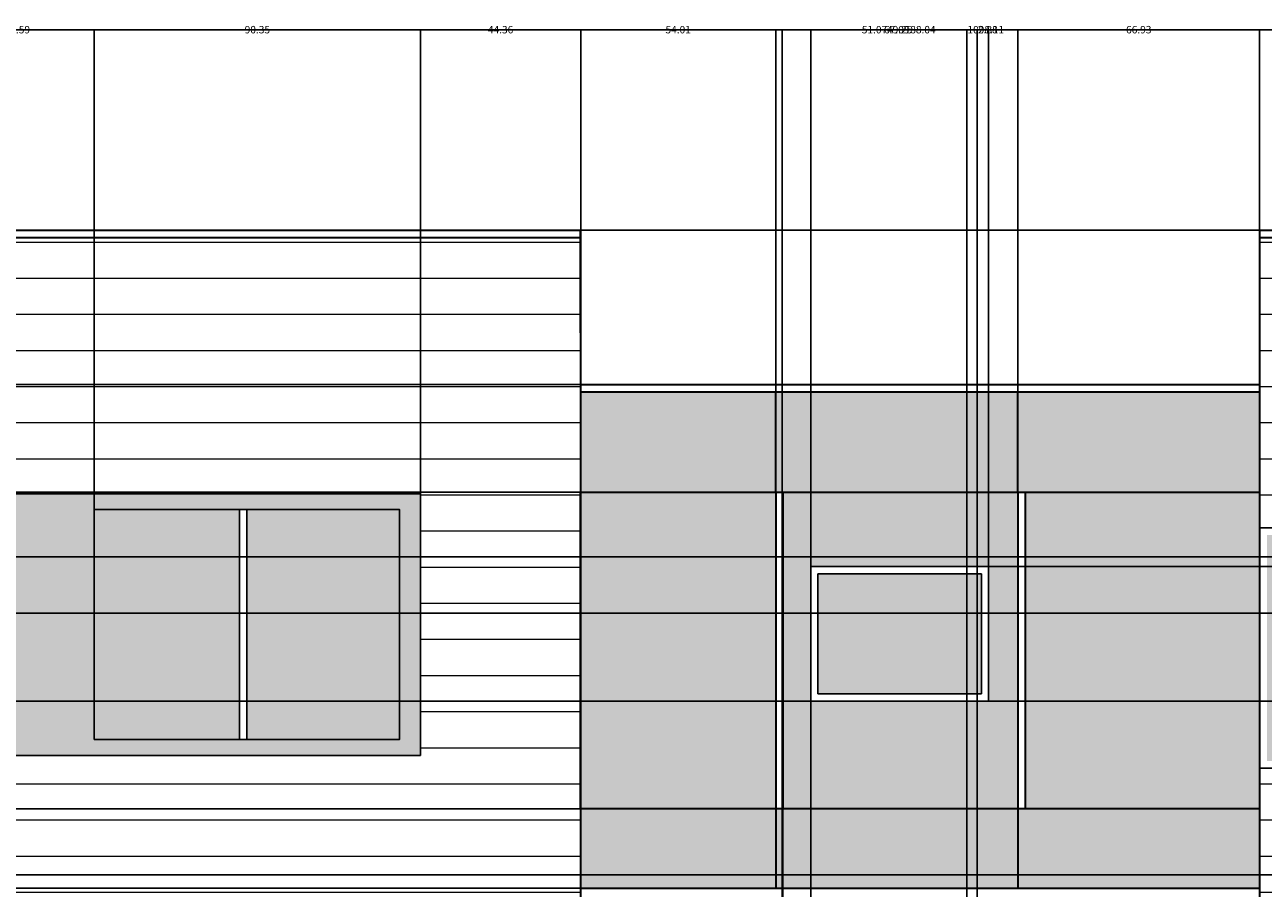
# Model space of a CAD drawing. Units: inches. Extents: x -30 to 1188, y 40 to 520.
# Tile 4 of 7: x 313 to 656, y 281 to 520. Entities that reach past the tile are written whole.
import ezdxf

# ---------------------------------------------------------------- set-up
doc = ezdxf.new("R2010")
doc.units = ezdxf.units.IN
doc.header["$MEASUREMENT"] = 0
for name, color, linetype, lineweight in [('A-ANNO-DIMS', 2, 'Continuous', 18), ('A-ELEV', 7, 'Continuous', 35), ('A-ELEV-PATT', 8, 'Continuous', 13), ('A-GLAZ', 4, 'Continuous', 25)]:
    doc.layers.add(name, color=color, linetype=linetype, lineweight=lineweight)
doc.styles.get("Standard").update_dxf_attribs({"font": 'arial.ttf'})
doc.dimstyles.get("Standard").update_dxf_attribs({"dimtxt": 2.0625, "dimasz": 0.18, "dimexe": 0.18, "dimexo": 0.0625, "dimgap": 0.09, "dimtad": 0, "dimtih": 1, "dimtoh": 1, "dimdec": 4, "dimzin": 0, "dimdsep": 46, "dimlunit": 4, "dimtxsty": 'Standard', "dimcen": 0.09, "dimadec": 0, "dimazin": 0, "dimtfac": 1, "dimtdec": 4, "dimtofl": 0, "dimtmove": 0, "dimatfit": 3, "dimfxl": 1, "dimtolj": 1, "dimtzin": 0, "dimarcsym": 0})

# ---------------------------------------------------------------- blocks, each defined once
blk = doc.blocks.new('WIN-SLIDING')
for p, q in [((40.27, 63.6), (40.27, 0)), ((42.27, 63.6), (42.27, 0))]:
    blk.add_line(p, q)
blk.add_lwpolyline([(0, 63.6), (84.55, 63.6), (84.55, 0), (0, 0)], close=True)
blk = doc.blocks.new('*D5')
at = {"layer": 'A-ANNO-DIMS', "color": 0, "lineweight": -2, "transparency": 16777216}
for p, q in [((73.66, 463.36), (73.66, 518.97)), ((73.84, 518.79), (266.76, 518.79)), ((466.82, 518.79), (273.9, 518.79)), ((467, 463.36), (467, 518.97))]:
    blk.add_line(p, q, dxfattribs=at)
at = {"layer": 'A-ANNO-DIMS', "color": 0, "transparency": 16777216}
for points in [[(73.84, 518.82), (73.84, 518.76), (73.66, 518.79)], [(466.82, 518.82), (466.82, 518.76), (467, 518.79)]]:
    blk.add_solid(points, dxfattribs=at)
at = {"layer": 'Defpoints', "color": 0, "transparency": 16777216}
for p in [(467, 518.79), (73.66, 463.29), (467, 463.29)]:
    blk.add_point(p, dxfattribs=at)
at = {"layer": 'A-ANNO-DIMS', "color": 0, "transparency": 16777216, "insert": (270.33, 518.79), "char_height": 2.062, "attachment_point": 5}
blk.add_mtext('\\A1;393.3', dxfattribs=at)
blk = doc.blocks.new('*D6')
at = {"layer": 'A-ANNO-DIMS', "color": 0, "lineweight": -2, "transparency": 16777216}
for p, q in [((467, 463.36), (467, 518.97)), ((467.18, 518.79), (556.74, 518.79)), ((654.85, 518.79), (565.28, 518.79)), ((655.03, 463.36), (655.03, 518.97))]:
    blk.add_line(p, q, dxfattribs=at)
at = {"layer": 'A-ANNO-DIMS', "color": 0, "transparency": 16777216}
for points in [[(467.18, 518.82), (467.18, 518.76), (467, 518.79)], [(654.85, 518.82), (654.85, 518.76), (655.03, 518.79)]]:
    blk.add_solid(points, dxfattribs=at)
at = {"layer": 'Defpoints', "color": 0, "transparency": 16777216}
for p in [(655.03, 518.79), (467, 463.29), (655.03, 463.29)]:
    blk.add_point(p, dxfattribs=at)
at = {"layer": 'A-ANNO-DIMS', "color": 0, "transparency": 16777216, "insert": (561.01, 518.79), "char_height": 2.062, "attachment_point": 5}
blk.add_mtext('\\A1;188.04', dxfattribs=at)
blk = doc.blocks.new('*D7')
at = {"layer": 'A-ANNO-DIMS', "color": 0, "lineweight": -2, "transparency": 16777216}
for p, q in [((655.03, 463.36), (655.03, 518.97)), ((655.21, 518.79), (791.88, 518.79)), ((935.72, 518.79), (799.06, 518.79)), ((935.9, 463.36), (935.9, 518.97))]:
    blk.add_line(p, q, dxfattribs=at)
at = {"layer": 'A-ANNO-DIMS', "color": 0, "transparency": 16777216}
for points in [[(655.21, 518.82), (655.21, 518.76), (655.03, 518.79)], [(935.72, 518.82), (935.72, 518.76), (935.9, 518.79)]]:
    blk.add_solid(points, dxfattribs=at)
at = {"layer": 'Defpoints', "color": 0, "transparency": 16777216}
for p in [(935.9, 518.79), (655.03, 463.29), (935.9, 463.29)]:
    blk.add_point(p, dxfattribs=at)
at = {"layer": 'A-ANNO-DIMS', "color": 0, "transparency": 16777216, "insert": (795.47, 518.79), "char_height": 2.062, "attachment_point": 5}
blk.add_mtext('\\A1;280.9', dxfattribs=at)
blk = doc.blocks.new('*D15')
at = {"layer": 'A-ANNO-DIMS', "color": 0, "lineweight": -2, "transparency": 16777216}
for p, q in [((289.7, 390.39), (289.7, 518.97)), ((289.88, 518.79), (307.38, 518.79)), ((332.11, 518.79), (314.61, 518.79)), ((332.29, 385.96), (332.29, 518.97))]:
    blk.add_line(p, q, dxfattribs=at)
at = {"layer": 'A-ANNO-DIMS', "color": 0, "transparency": 16777216}
for points in [[(289.88, 518.82), (289.88, 518.76), (289.7, 518.79)], [(332.11, 518.82), (332.11, 518.76), (332.29, 518.79)]]:
    blk.add_solid(points, dxfattribs=at)
at = {"layer": 'Defpoints', "color": 0, "transparency": 16777216}
for p in [(332.29, 518.79), (289.7, 390.32), (332.29, 385.9)]:
    blk.add_point(p, dxfattribs=at)
at = {"layer": 'A-ANNO-DIMS', "color": 0, "transparency": 16777216, "insert": (310.99, 518.79), "char_height": 2.062, "attachment_point": 5}
blk.add_mtext('\\A1;42.59', dxfattribs=at)
blk = doc.blocks.new('*D16')
at = {"layer": 'A-ANNO-DIMS', "color": 0, "lineweight": -2, "transparency": 16777216}
for p, q in [((332.29, 385.96), (332.29, 518.97)), ((332.47, 518.79), (373.89, 518.79)), ((422.46, 518.79), (381.04, 518.79)), ((422.64, 390.39), (422.64, 518.97))]:
    blk.add_line(p, q, dxfattribs=at)
at = {"layer": 'A-ANNO-DIMS', "color": 0, "transparency": 16777216}
for points in [[(332.47, 518.82), (332.47, 518.76), (332.29, 518.79)], [(422.46, 518.82), (422.46, 518.76), (422.64, 518.79)]]:
    blk.add_solid(points, dxfattribs=at)
at = {"layer": 'Defpoints', "color": 0, "transparency": 16777216}
for p in [(422.64, 518.79), (422.64, 390.32), (332.29, 385.9)]:
    blk.add_point(p, dxfattribs=at)
at = {"layer": 'A-ANNO-DIMS', "color": 0, "transparency": 16777216, "insert": (377.46, 518.79), "char_height": 2.062, "attachment_point": 5}
blk.add_mtext('\\A1;90.35', dxfattribs=at)
blk = doc.blocks.new('*D17')
at = {"layer": 'A-ANNO-DIMS', "color": 0, "lineweight": -2, "transparency": 16777216}
for p, q in [((422.64, 390.39), (422.64, 518.97)), ((422.82, 518.79), (441.21, 518.79)), ((466.82, 518.79), (448.43, 518.79)), ((467, 390.84), (467, 518.97))]:
    blk.add_line(p, q, dxfattribs=at)
at = {"layer": 'A-ANNO-DIMS', "color": 0, "transparency": 16777216}
for points in [[(422.82, 518.82), (422.82, 518.76), (422.64, 518.79)], [(466.82, 518.82), (466.82, 518.76), (467, 518.79)]]:
    blk.add_solid(points, dxfattribs=at)
at = {"layer": 'Defpoints', "color": 0, "transparency": 16777216}
for p in [(467, 518.79), (422.64, 390.32), (467, 390.77)]:
    blk.add_point(p, dxfattribs=at)
at = {"layer": 'A-ANNO-DIMS', "color": 0, "transparency": 16777216, "insert": (444.82, 518.79), "char_height": 2.062, "attachment_point": 5}
blk.add_mtext('\\A1;44.36', dxfattribs=at)
blk = doc.blocks.new('*D24')
at = {"layer": 'A-ANNO-DIMS', "color": 0, "lineweight": -2, "transparency": 16777216}
for p, q in [((935.84, 463.29), (-25.83, 463.29)), ((-25.65, 463.11), (-25.65, 419.2)), ((-25.65, 373.01), (-25.65, 416.92)), ((980.66, 372.83), (-25.83, 372.83))]:
    blk.add_line(p, q, dxfattribs=at)
at = {"layer": 'A-ANNO-DIMS', "color": 0, "transparency": 16777216}
for points in [[(-25.68, 463.11), (-25.62, 463.11), (-25.65, 463.29)], [(-25.68, 373.01), (-25.62, 373.01), (-25.65, 372.83)]]:
    blk.add_solid(points, dxfattribs=at)
at = {"layer": 'Defpoints', "color": 0, "transparency": 16777216}
for p in [(-25.65, 463.29), (935.9, 463.29), (980.73, 372.83)]:
    blk.add_point(p, dxfattribs=at)
at = {"layer": 'A-ANNO-DIMS', "color": 0, "transparency": 16777216, "insert": (-25.65, 418.06), "char_height": 2.062, "attachment_point": 5}
blk.add_mtext('\\A1;90.47', dxfattribs=at)
blk = doc.blocks.new('*D25')
at = {"layer": 'A-ANNO-DIMS', "color": 0, "lineweight": -2, "transparency": 16777216}
for p, q in [((655.03, 380.92), (655.03, 518.97)), ((655.21, 518.79), (722.39, 518.79)), ((798.12, 518.79), (730.94, 518.79)), ((798.3, 380.92), (798.3, 518.97))]:
    blk.add_line(p, q, dxfattribs=at)
at = {"layer": 'A-ANNO-DIMS', "color": 0, "transparency": 16777216}
for points in [[(655.21, 518.82), (655.21, 518.76), (655.03, 518.79)], [(798.12, 518.82), (798.12, 518.76), (798.3, 518.79)]]:
    blk.add_solid(points, dxfattribs=at)
at = {"layer": 'Defpoints', "color": 0, "transparency": 16777216}
for p in [(798.3, 518.79), (655.03, 380.86), (798.3, 380.86)]:
    blk.add_point(p, dxfattribs=at)
at = {"layer": 'A-ANNO-DIMS', "color": 0, "transparency": 16777216, "insert": (726.67, 518.79), "char_height": 2.062, "attachment_point": 5}
blk.add_mtext('\\A1;143.27', dxfattribs=at)
blk = doc.blocks.new('*D41')
at = {"layer": 'A-ANNO-DIMS', "color": 0, "lineweight": -2, "transparency": 16777216}
for p, q in [((654.97, 463.29), (-25.83, 463.29)), ((-25.65, 463.11), (-25.65, 443.04)), ((-25.65, 420.69), (-25.65, 440.76)), ((654.97, 420.51), (-25.83, 420.51))]:
    blk.add_line(p, q, dxfattribs=at)
at = {"layer": 'A-ANNO-DIMS', "color": 0, "transparency": 16777216}
for points in [[(-25.68, 463.11), (-25.62, 463.11), (-25.65, 463.29)], [(-25.68, 420.69), (-25.62, 420.69), (-25.65, 420.51)]]:
    blk.add_solid(points, dxfattribs=at)
at = {"layer": 'Defpoints', "color": 0, "transparency": 16777216}
for p in [(655.03, 463.29), (-25.65, 420.51), (655.03, 420.51)]:
    blk.add_point(p, dxfattribs=at)
at = {"layer": 'A-ANNO-DIMS', "color": 0, "transparency": 16777216, "insert": (-25.65, 441.9), "char_height": 2.062, "attachment_point": 5}
blk.add_mtext('\\A1;42.785', dxfattribs=at)
blk = doc.blocks.new('*D45')
at = {"layer": 'A-ANNO-DIMS', "color": 0, "lineweight": -2, "transparency": 16777216}
for p, q in [((945.03, 284.84), (-25.83, 284.84)), ((-25.65, 284.66), (-25.65, 273.81)), ((-25.65, 260.67), (-25.65, 271.52)), ((935.84, 260.49), (-25.83, 260.49))]:
    blk.add_line(p, q, dxfattribs=at)
at = {"layer": 'A-ANNO-DIMS', "color": 0, "transparency": 16777216}
for points in [[(-25.68, 284.66), (-25.62, 284.66), (-25.65, 284.84)], [(-25.68, 260.67), (-25.62, 260.67), (-25.65, 260.49)]]:
    blk.add_solid(points, dxfattribs=at)
at = {"layer": 'Defpoints', "color": 0, "transparency": 16777216}
for p in [(945.1, 284.84), (-25.65, 260.49), (935.9, 260.49)]:
    blk.add_point(p, dxfattribs=at)
at = {"layer": 'A-ANNO-DIMS', "color": 0, "transparency": 16777216, "insert": (-25.65, 272.67), "char_height": 2.062, "attachment_point": 5}
blk.add_mtext('\\A1;24.35', dxfattribs=at)
blk = doc.blocks.new('*D46')
at = {"layer": 'A-ANNO-DIMS', "color": 0, "lineweight": -2, "transparency": 16777216}
for p, q in [((945.03, 357.27), (-25.83, 357.27)), ((-25.65, 357.09), (-25.65, 322.2)), ((-25.65, 285.02), (-25.65, 319.91)), ((945.03, 284.84), (-25.83, 284.84))]:
    blk.add_line(p, q, dxfattribs=at)
at = {"layer": 'A-ANNO-DIMS', "color": 0, "transparency": 16777216}
for points in [[(-25.68, 357.09), (-25.62, 357.09), (-25.65, 357.27)], [(-25.68, 285.02), (-25.62, 285.02), (-25.65, 284.84)]]:
    blk.add_solid(points, dxfattribs=at)
at = {"layer": 'Defpoints', "color": 0, "transparency": 16777216}
for p in [(-25.65, 357.27), (945.1, 357.27), (945.1, 284.84)]:
    blk.add_point(p, dxfattribs=at)
at = {"layer": 'A-ANNO-DIMS', "color": 0, "transparency": 16777216, "insert": (-25.65, 321.06), "char_height": 2.062, "attachment_point": 5}
blk.add_mtext('\\A1;72.43', dxfattribs=at)
blk = doc.blocks.new('*D47')
at = {"layer": 'A-ANNO-DIMS', "color": 0, "lineweight": -2, "transparency": 16777216}
for p, q in [((935.84, 372.83), (-25.83, 372.83)), ((-25.65, 372.65), (-25.65, 366.19)), ((-25.65, 357.45), (-25.65, 363.91)), ((945.03, 357.27), (-25.83, 357.27))]:
    blk.add_line(p, q, dxfattribs=at)
at = {"layer": 'A-ANNO-DIMS', "color": 0, "transparency": 16777216}
for points in [[(-25.68, 372.65), (-25.62, 372.65), (-25.65, 372.83)], [(-25.68, 357.45), (-25.62, 357.45), (-25.65, 357.27)]]:
    blk.add_solid(points, dxfattribs=at)
at = {"layer": 'Defpoints', "color": 0, "transparency": 16777216}
for p in [(-25.65, 372.83), (935.9, 372.83), (945.1, 357.27)]:
    blk.add_point(p, dxfattribs=at)
at = {"layer": 'A-ANNO-DIMS', "color": 0, "transparency": 16777216, "insert": (-25.65, 365.05), "char_height": 2.062, "attachment_point": 5}
blk.add_mtext('\\A1;15.554', dxfattribs=at)
blk = doc.blocks.new('*D58')
at = {"layer": 'A-ANNO-DIMS', "color": 0, "lineweight": -2, "transparency": 16777216}
for p, q in [((466.93, 303.05), (-25.83, 303.05)), ((-25.65, 302.87), (-25.65, 293.22)), ((-25.65, 281.27), (-25.65, 290.93)), ((466.93, 281.09), (-25.83, 281.09))]:
    blk.add_line(p, q, dxfattribs=at)
at = {"layer": 'A-ANNO-DIMS', "color": 0, "transparency": 16777216}
for points in [[(-25.68, 302.87), (-25.62, 302.87), (-25.65, 303.05)], [(-25.68, 281.27), (-25.62, 281.27), (-25.65, 281.09)]]:
    blk.add_solid(points, dxfattribs=at)
at = {"layer": 'Defpoints', "color": 0, "transparency": 16777216}
for p in [(-25.65, 303.05), (467, 303.05), (467, 281.09)]:
    blk.add_point(p, dxfattribs=at)
at = {"layer": 'A-ANNO-DIMS', "color": 0, "transparency": 16777216, "insert": (-25.65, 292.07), "char_height": 2.062, "attachment_point": 5}
blk.add_mtext('\\A1;21.96', dxfattribs=at)
blk = doc.blocks.new('*D59')
at = {"layer": 'A-ANNO-DIMS', "color": 0, "lineweight": -2, "transparency": 16777216}
for p, q in [((466.93, 390.77), (-25.83, 390.77)), ((-25.65, 390.59), (-25.65, 348.06)), ((-25.65, 303.23), (-25.65, 345.77)), ((466.93, 303.05), (-25.83, 303.05))]:
    blk.add_line(p, q, dxfattribs=at)
at = {"layer": 'A-ANNO-DIMS', "color": 0, "transparency": 16777216}
for points in [[(-25.68, 390.59), (-25.62, 390.59), (-25.65, 390.77)], [(-25.68, 303.23), (-25.62, 303.23), (-25.65, 303.05)]]:
    blk.add_solid(points, dxfattribs=at)
at = {"layer": 'Defpoints', "color": 0, "transparency": 16777216}
for p in [(-25.65, 390.77), (467, 390.77), (467, 303.05)]:
    blk.add_point(p, dxfattribs=at)
at = {"layer": 'A-ANNO-DIMS', "color": 0, "transparency": 16777216, "insert": (-25.65, 346.91), "char_height": 2.062, "attachment_point": 5}
blk.add_mtext('\\A1;87.72', dxfattribs=at)
blk = doc.blocks.new('*D60')
at = {"layer": 'A-ANNO-DIMS', "color": 0, "lineweight": -2, "transparency": 16777216}
for p, q in [((466.93, 420.51), (-25.83, 420.51)), ((-25.65, 420.33), (-25.65, 406.78)), ((-25.65, 390.95), (-25.65, 404.5)), ((466.93, 390.77), (-25.83, 390.77))]:
    blk.add_line(p, q, dxfattribs=at)
at = {"layer": 'A-ANNO-DIMS', "color": 0, "transparency": 16777216}
for points in [[(-25.68, 420.33), (-25.62, 420.33), (-25.65, 420.51)], [(-25.68, 390.95), (-25.62, 390.95), (-25.65, 390.77)]]:
    blk.add_solid(points, dxfattribs=at)
at = {"layer": 'Defpoints', "color": 0, "transparency": 16777216}
for p in [(-25.65, 420.51), (467, 420.51), (467, 390.77)]:
    blk.add_point(p, dxfattribs=at)
at = {"layer": 'A-ANNO-DIMS', "color": 0, "transparency": 16777216, "insert": (-25.65, 405.64), "char_height": 2.062, "attachment_point": 5}
blk.add_mtext('\\A1;29.735', dxfattribs=at)
blk = doc.blocks.new('*D65')
at = {"layer": 'A-ANNO-DIMS', "color": 0, "lineweight": -2, "transparency": 16777216}
for p, q in [((522.84, 271.44), (522.84, 518.97)), ((523.02, 518.79), (544.8, 518.79)), ((573.72, 518.79), (551.94, 518.79)), ((573.9, 245.23), (573.9, 518.97))]:
    blk.add_line(p, q, dxfattribs=at)
at = {"layer": 'A-ANNO-DIMS', "color": 0, "transparency": 16777216}
for points in [[(523.02, 518.82), (523.02, 518.76), (522.84, 518.79)], [(573.72, 518.82), (573.72, 518.76), (573.9, 518.79)]]:
    blk.add_solid(points, dxfattribs=at)
at = {"layer": 'Defpoints', "color": 0, "transparency": 16777216}
for p in [(522.84, 518.79), (522.84, 271.38), (573.9, 245.17)]:
    blk.add_point(p, dxfattribs=at)
at = {"layer": 'A-ANNO-DIMS', "color": 0, "transparency": 16777216, "insert": (548.37, 518.79), "char_height": 2.062, "attachment_point": 5}
blk.add_mtext('\\A1;51.07', dxfattribs=at)
blk = doc.blocks.new('*D66')
at = {"layer": 'A-ANNO-DIMS', "color": 0, "lineweight": -2, "transparency": 16777216}
for p, q in [((573.9, 245.23), (573.9, 518.97)), ((574.08, 518.79), (576.6, 518.79)), ((576.78, 245.23), (576.78, 518.97)), ((576.78, 518.79), (576.96, 518.79))]:
    blk.add_line(p, q, dxfattribs=at)
at = {"layer": 'A-ANNO-DIMS', "color": 0, "transparency": 16777216}
for points in [[(574.08, 518.82), (574.08, 518.76), (573.9, 518.79)], [(576.6, 518.82), (576.6, 518.76), (576.78, 518.79)]]:
    blk.add_solid(points, dxfattribs=at)
at = {"layer": 'Defpoints', "color": 0, "transparency": 16777216}
for p in [(576.78, 518.79), (573.9, 245.17), (576.78, 245.17)]:
    blk.add_point(p, dxfattribs=at)
at = {"layer": 'A-ANNO-DIMS', "color": 0, "transparency": 16777216, "insert": (579.75, 518.79), "char_height": 2.062, "attachment_point": 5}
blk.add_mtext('\\A1;2.88', dxfattribs=at)
blk = doc.blocks.new('*D67')
at = {"layer": 'A-ANNO-DIMS', "color": 0, "lineweight": -2, "transparency": 16777216}
for p, q in [((530.73, 370.19), (530.73, 518.97)), ((530.91, 518.79), (551.73, 518.79)), ((579.79, 518.79), (558.97, 518.79)), ((579.97, 370.19), (579.97, 518.97))]:
    blk.add_line(p, q, dxfattribs=at)
at = {"layer": 'A-ANNO-DIMS', "color": 0, "transparency": 16777216}
for points in [[(530.91, 518.82), (530.91, 518.76), (530.73, 518.79)], [(579.79, 518.82), (579.79, 518.76), (579.97, 518.79)]]:
    blk.add_solid(points, dxfattribs=at)
at = {"layer": 'Defpoints', "color": 0, "transparency": 16777216}
for p in [(579.97, 518.79), (530.73, 370.13), (579.97, 370.13)]:
    blk.add_point(p, dxfattribs=at)
at = {"layer": 'A-ANNO-DIMS', "color": 0, "transparency": 16777216, "insert": (555.35, 518.79), "char_height": 2.062, "attachment_point": 5}
blk.add_mtext('\\A1;49.25', dxfattribs=at)
blk = doc.blocks.new('*D68')
at = {"layer": 'A-ANNO-DIMS', "color": 0, "lineweight": -2, "transparency": 16777216}
for p, q in [((580.04, 370.13), (1183.93, 370.13)), ((1183.75, 369.95), (1183.75, 352.67)), ((1183.75, 333.09), (1183.75, 350.38)), ((580.04, 332.91), (1183.93, 332.91))]:
    blk.add_line(p, q, dxfattribs=at)
at = {"layer": 'A-ANNO-DIMS', "color": 0, "transparency": 16777216}
for points in [[(1183.72, 369.95), (1183.78, 369.95), (1183.75, 370.13)], [(1183.72, 333.09), (1183.78, 333.09), (1183.75, 332.91)]]:
    blk.add_solid(points, dxfattribs=at)
at = {"layer": 'Defpoints', "color": 0, "transparency": 16777216}
for p in [(579.97, 370.13), (1183.75, 370.13), (579.97, 332.91)]:
    blk.add_point(p, dxfattribs=at)
at = {"layer": 'A-ANNO-DIMS', "color": 0, "transparency": 16777216, "insert": (1183.75, 351.52), "char_height": 2.062, "attachment_point": 5}
blk.add_mtext('\\A1;37.22', dxfattribs=at)
blk = doc.blocks.new('*D69')
at = {"layer": 'A-ANNO-DIMS', "color": 0, "lineweight": -2, "transparency": 16777216}
for p, q in [((530.66, 332.91), (-25.83, 332.91)), ((-25.65, 332.73), (-25.65, 319.13)), ((-25.65, 303.23), (-25.65, 316.84)), ((520.94, 303.05), (-25.83, 303.05))]:
    blk.add_line(p, q, dxfattribs=at)
at = {"layer": 'A-ANNO-DIMS', "color": 0, "transparency": 16777216}
for points in [[(-25.68, 332.73), (-25.62, 332.73), (-25.65, 332.91)], [(-25.68, 303.23), (-25.62, 303.23), (-25.65, 303.05)]]:
    blk.add_solid(points, dxfattribs=at)
at = {"layer": 'Defpoints', "color": 0, "transparency": 16777216}
for p in [(-25.65, 332.91), (530.73, 332.91), (521.01, 303.05)]:
    blk.add_point(p, dxfattribs=at)
at = {"layer": 'A-ANNO-DIMS', "color": 0, "transparency": 16777216, "insert": (-25.65, 317.98), "char_height": 2.062, "attachment_point": 5}
blk.add_mtext('\\A1;29.86', dxfattribs=at)
blk = doc.blocks.new('*D70')
at = {"layer": 'A-ANNO-DIMS', "color": 0, "lineweight": -2, "transparency": 16777216}
for p, q in [((530.73, 332.85), (530.73, 41.19)), ((523.01, 302.99), (523.01, 41.19)), ((523.19, 41.37), (523.3, 41.37)), ((530.55, 41.37), (530.43, 41.37))]:
    blk.add_line(p, q, dxfattribs=at)
at = {"layer": 'A-ANNO-DIMS', "color": 0, "transparency": 16777216}
for points in [[(523.19, 41.4), (523.19, 41.34), (523.01, 41.37)], [(530.55, 41.4), (530.55, 41.34), (530.73, 41.37)]]:
    blk.add_solid(points, dxfattribs=at)
at = {"layer": 'Defpoints', "color": 0, "transparency": 16777216}
for p in [(530.73, 332.91), (523.01, 303.05), (523.01, 41.37)]:
    blk.add_point(p, dxfattribs=at)
at = {"layer": 'A-ANNO-DIMS', "color": 0, "transparency": 16777216, "insert": (526.87, 41.37), "char_height": 2.062, "attachment_point": 5}
blk.add_mtext('\\A1;7.718', dxfattribs=at)
blk = doc.blocks.new('*D71')
at = {"layer": 'A-ANNO-DIMS', "color": 0, "lineweight": -2, "transparency": 16777216}
for p, q in [((467, 418.57), (467, 518.97)), ((467.18, 518.79), (490.63, 518.79)), ((520.83, 518.79), (497.37, 518.79)), ((521.01, 418.57), (521.01, 518.97))]:
    blk.add_line(p, q, dxfattribs=at)
at = {"layer": 'A-ANNO-DIMS', "color": 0, "transparency": 16777216}
for points in [[(467.18, 518.82), (467.18, 518.76), (467, 518.79)], [(520.83, 518.82), (520.83, 518.76), (521.01, 518.79)]]:
    blk.add_solid(points, dxfattribs=at)
at = {"layer": 'Defpoints', "color": 0, "transparency": 16777216}
for p in [(521.01, 518.79), (467, 418.51), (521.01, 418.51)]:
    blk.add_point(p, dxfattribs=at)
at = {"layer": 'A-ANNO-DIMS', "color": 0, "transparency": 16777216, "insert": (494, 518.79), "char_height": 2.062, "attachment_point": 5}
blk.add_mtext('\\A1;54.01', dxfattribs=at)
blk = doc.blocks.new('*D72')
at = {"layer": 'A-ANNO-DIMS', "color": 0, "lineweight": -2, "transparency": 16777216}
for p, q in [((521.01, 418.57), (521.01, 518.97)), ((521.19, 518.79), (550.97, 518.79)), ((587.92, 518.79), (558.13, 518.79)), ((588.1, 418.57), (588.1, 518.97))]:
    blk.add_line(p, q, dxfattribs=at)
at = {"layer": 'A-ANNO-DIMS', "color": 0, "transparency": 16777216}
for points in [[(521.19, 518.82), (521.19, 518.76), (521.01, 518.79)], [(587.92, 518.82), (587.92, 518.76), (588.1, 518.79)]]:
    blk.add_solid(points, dxfattribs=at)
at = {"layer": 'Defpoints', "color": 0, "transparency": 16777216}
for p in [(588.1, 518.79), (521.01, 418.51), (588.1, 418.51)]:
    blk.add_point(p, dxfattribs=at)
at = {"layer": 'A-ANNO-DIMS', "color": 0, "transparency": 16777216, "insert": (554.55, 518.79), "char_height": 2.062, "attachment_point": 5}
blk.add_mtext('\\A1;67.09', dxfattribs=at)
blk = doc.blocks.new('*D73')
at = {"layer": 'A-ANNO-DIMS', "color": 0, "lineweight": -2, "transparency": 16777216}
for p, q in [((588.1, 418.57), (588.1, 518.97)), ((588.28, 518.79), (617.99, 518.79)), ((654.85, 518.79), (625.14, 518.79)), ((655.03, 418.57), (655.03, 518.97))]:
    blk.add_line(p, q, dxfattribs=at)
at = {"layer": 'A-ANNO-DIMS', "color": 0, "transparency": 16777216}
for points in [[(588.28, 518.82), (588.28, 518.76), (588.1, 518.79)], [(654.85, 518.82), (654.85, 518.76), (655.03, 518.79)]]:
    blk.add_solid(points, dxfattribs=at)
at = {"layer": 'Defpoints', "color": 0, "transparency": 16777216}
for p in [(655.03, 518.79), (588.1, 418.51), (655.03, 418.51)]:
    blk.add_point(p, dxfattribs=at)
at = {"layer": 'A-ANNO-DIMS', "color": 0, "transparency": 16777216, "insert": (621.56, 518.79), "char_height": 2.062, "attachment_point": 5}
blk.add_mtext('\\A1;66.93', dxfattribs=at)
blk = doc.blocks.new('*D74')
at = {"layer": 'A-ANNO-DIMS', "color": 0, "lineweight": -2, "transparency": 16777216}
for p, q in [((30.14, 98.93), (30.14, 518.97)), ((30.32, 518.79), (574.32, 518.79)), ((1128.07, 518.79), (584.07, 518.79)), ((1128.25, 117.62), (1128.25, 518.97))]:
    blk.add_line(p, q, dxfattribs=at)
at = {"layer": 'A-ANNO-DIMS', "color": 0, "transparency": 16777216}
for points in [[(30.32, 518.82), (30.32, 518.76), (30.14, 518.79)], [(1128.07, 518.82), (1128.07, 518.76), (1128.25, 518.79)]]:
    blk.add_solid(points, dxfattribs=at)
at = {"layer": 'Defpoints', "color": 0, "transparency": 16777216}
for p in [(1128.25, 518.79), (1128.25, 117.56), (30.14, 98.87)]:
    blk.add_point(p, dxfattribs=at)
at = {"layer": 'A-ANNO-DIMS', "color": 0, "transparency": 16777216, "insert": (579.19, 518.79), "char_height": 2.0625, "attachment_point": 5}
blk.add_mtext('\\A1;1098.11', dxfattribs=at)

msp = doc.modelspace()

# ---------------------------------------------------------------- hatches: boundary and pattern name
at = {"layer": 'A-ELEV-PATT'}
h = msp.add_hatch(dxfattribs=at)
h.set_pattern_fill('ANSI31', color=256, scale=80, angle=135)
h.paths.add_polyline_path([(935.904, 461.2934), (655.0318, 461.2934), (655.0318, 408.0708), (655.0318, 380.8615), (798.3036, 380.8615), (798.3036, 314.3348), (655.0318, 314.3348), (655.0318, 303.0545), (655.0318, 122.8714), (744.4225, 122.8714), (796.5546, 122.8714), (935.904, 122.8714), (935.904, 203.8438), (792.6322, 203.8438), (792.6322, 270.3705), (935.904, 270.3705), (935.904, 372.8284)])
h.paths.add_polyline_path([(466.9951, 434.8714), (466.9951, 461.2934), (73.6582, 461.2934), (73.6582, 434.8714), (73.6582, 410.8714), (73.6582, 266.8714), (382.4247, 266.8714), (466.9951, 266.8714)])
h.paths.add_polyline_path([(422.6392, 390.3227), (422.6392, 317.8826), (99.4312, 317.8826), (99.4312, 390.3227)], flags=16)
h.paths.add_polyline_path([(416.8376, 385.9009), (416.8376, 322.3026), (332.2885, 322.3026), (332.2885, 385.9009)], flags=0)
h.paths.add_polyline_path([(187.4151, 386.0591), (187.4151, 322.4608), (102.866, 322.4608), (102.866, 386.0591)], flags=0)
h = msp.add_hatch(color=256, dxfattribs=at)
h.dxf.hatch_style = 1
h.paths.add_polyline_path([(99.4312, 186.9265), (73.6582, 186.9265), (73.6582, 133.1393), (99.4312, 133.1393)])
h.paths.add_polyline_path([(99.4312, 242.8714), (73.6582, 242.8714), (73.6582, 186.9265), (99.4312, 186.9265)])
h.paths.add_polyline_path([(99.4312, 266.8714), (73.6582, 266.8714), (73.6582, 242.8714), (99.4312, 242.8714)])
h.paths.add_polyline_path([(244.2768, 266.8714), (99.4312, 266.8714), (99.4312, 242.8714), (130.129, 242.8714), (244.2768, 242.8714)])
h.paths.add_polyline_path([(358.4247, 266.8714), (244.2768, 266.8714), (244.2768, 242.8714), (358.4247, 242.8714)])
h.paths.add_polyline_path([(466.8255, 266.8714), (382.4247, 266.8714), (358.4247, 266.8714), (358.4247, 242.8714), (382.4247, 242.8714), (466.8255, 242.8714)])
h.paths.add_polyline_path([(466.8255, 242.8714), (382.4247, 242.8714), (358.4247, 242.8714), (358.4247, 186.9265), (382.4247, 186.9265), (466.8255, 186.9265)])
h.paths.add_polyline_path([(466.8255, 186.9265), (382.4247, 186.9265), (358.4247, 186.9265), (358.4247, 133.1393), (382.4247, 133.1393), (466.9951, 133.1393), (466.9951, 140.7981), (466.8255, 140.7981)])
h.paths.add_polyline_path([(521.0073, 303.0545), (466.9951, 303.0545), (466.9951, 281.0934), (521.0073, 281.0934)])
h.paths.add_polyline_path([(588.0971, 303.0545), (521.0073, 303.0545), (521.0073, 281.0934), (588.0971, 281.0934)])
h.paths.add_polyline_path([(655.0318, 303.0545), (588.0971, 303.0545), (588.0971, 281.0934), (655.0318, 281.0934)])
h.paths.add_polyline_path([(655.0318, 408.0708), (655.0318, 418.5083), (588.0971, 418.5083), (588.0971, 390.7733), (655.0318, 390.7733)])
h.paths.add_polyline_path([(588.0971, 418.5083), (521.0073, 418.5083), (521.0073, 390.7733), (588.0971, 390.7733)])
h.paths.add_polyline_path([(521.0073, 418.5083), (466.9951, 418.5083), (466.9951, 390.7733), (521.0073, 390.7733)])
h = msp.add_hatch(color=256, dxfattribs=at)
h.dxf.hatch_style = 1
h.paths.add_polyline_path([(521.0073, 390.7733), (466.9951, 390.7733), (466.9951, 303.0545), (521.0073, 303.0545)])
h.paths.add_polyline_path([(588.0971, 390.7733), (523.0073, 390.7733), (523.0073, 303.0545), (588.0971, 303.0545)])
h.paths.add_polyline_path([(579.9749, 370.1304), (579.9749, 332.9128), (530.7254, 332.9128), (530.7254, 370.1304)], flags=16)
h.paths.add_polyline_path([(577.9749, 368.1304), (577.9749, 334.9128), (532.7254, 334.9128), (532.7254, 368.1304)], flags=0)
h.paths.add_polyline_path([(655.0318, 390.7733), (590.0971, 390.7733), (590.0971, 303.0545), (655.0318, 303.0545)])
h.paths.add_polyline_path([(577.9749, 368.1304), (532.7254, 368.1304), (532.7254, 334.9128), (577.9749, 334.9128)], flags=0)
h.paths.add_polyline_path([(416.8376, 385.9009), (374.5631, 385.9009), (374.5631, 322.3026), (416.8376, 322.3026)])
h.paths.add_polyline_path([(372.5631, 385.9009), (332.2885, 385.9009), (332.2885, 322.3026), (372.5631, 322.3026)])
h.paths.add_polyline_path([(187.4151, 386.0591), (102.866, 386.0591), (102.866, 322.4608), (187.4151, 322.4608)])
h.paths.add_polyline_path([(697.0557, 378.8615), (657.0318, 378.8615), (657.0318, 316.3348), (697.0557, 316.3348)])
h.paths.add_polyline_path([(746.916, 378.8615), (699.0557, 378.8615), (699.0557, 316.3348), (746.916, 316.3348)])
h.paths.add_polyline_path([(796.3036, 378.8615), (748.916, 378.8615), (748.916, 316.3348), (796.3036, 316.3348)])
h.paths.add_polyline_path([(884.5164, 268.3705), (836.6561, 268.3705), (836.6561, 205.8438), (884.5164, 205.8438)])
h.paths.add_polyline_path([(834.6561, 268.3705), (794.6322, 268.3705), (794.6322, 205.8438), (834.6561, 205.8438)])
h.paths.add_polyline_path([(967.928, 357.2748), (945.0964, 357.2748), (945.0964, 284.8425), (967.928, 284.8425)])
h = msp.add_hatch(color=256, dxfattribs=at)
h.dxf.hatch_style = 1
h.paths.add_polyline_path([(237.1312, 390.3227), (187.4151, 390.3227), (187.4151, 386.0591), (187.4151, 322.4608), (187.4151, 317.8826), (237.1312, 317.8826)])
h.paths.add_polyline_path([(289.6973, 390.3227), (237.1312, 390.3227), (237.1312, 317.8826), (289.6973, 317.8826)])
h.paths.add_polyline_path([(422.6392, 390.3227), (289.6973, 390.3227), (289.6973, 317.8826), (422.6392, 317.8826)])
h.paths.add_polyline_path([(332.2885, 385.9009), (416.8376, 385.9009), (416.8376, 322.3026), (332.2885, 322.3026)], flags=16)
h.paths.add_polyline_path([(520.8377, 255.4488), (468.8255, 255.4488), (468.8255, 208.218), (520.8377, 208.218)])
h.paths.add_polyline_path([(573.9028, 245.1654), (576.7826, 245.1654), (576.7826, 208.218), (587.9675, 208.218), (587.9675, 255.4488), (522.8377, 255.4488), (522.8377, 208.218), (573.9028, 208.218)])
h.paths.add_polyline_path([(652.8622, 255.4488), (589.9675, 255.4488), (589.9675, 208.218), (652.8622, 208.218)])
h.paths.add_polyline_path([(652.8622, 206.218), (589.9675, 206.218), (589.9675, 142.7981), (652.8622, 142.7981)])
h.paths.add_polyline_path([(573.9028, 206.218), (522.8377, 206.218), (522.8377, 142.7981), (587.9675, 142.7981), (587.9675, 206.218), (576.7826, 206.218), (576.7826, 153.0843), (573.9028, 153.0843)])
h.paths.add_polyline_path([(520.8377, 206.218), (468.8255, 206.218), (468.8255, 142.7981), (520.8377, 142.7981)])
h.paths.add_polyline_path([(520.8377, 271.3754), (468.8255, 271.3754), (468.8255, 255.4488), (520.8377, 255.4488)])
h.paths.add_polyline_path([(587.9675, 271.3754), (522.8377, 271.3754), (522.8377, 255.4488), (587.9675, 255.4488)])
h.paths.add_polyline_path([(652.8622, 271.3754), (589.9675, 271.3754), (589.9675, 255.4488), (652.8622, 255.4488)])
h.paths.add_polyline_path([(935.904, 270.3705), (886.5164, 270.3705), (886.5164, 268.3705), (886.5164, 205.8438), (886.5164, 203.8438), (935.904, 203.8438)])
h.paths.add_polyline_path([(978.7252, 275.3408), (937.904, 275.3408), (937.904, 262.4906), (978.7252, 262.4906)])
h.paths.add_polyline_path([(978.7252, 370.8284), (937.904, 370.8284), (937.904, 275.3408), (978.7252, 275.3408)])
h.paths.add_polyline_path([(967.928, 284.8425), (945.0964, 284.8425), (945.0964, 357.2748), (967.928, 357.2748)], flags=16)
h = msp.add_hatch(color=256, dxfattribs=at)
h.dxf.hatch_style = 1
h.paths.add_polyline_path([(577.9749, 368.1304), (532.7254, 368.1304), (532.7254, 334.9128), (577.9749, 334.9128)])

# ---------------------------------------------------------------- linework, layer by layer
at = {"layer": 'A-ELEV'}
for p, q in [((73.6582, 463.2934), (466.9951, 463.2934)), ((466.9951, 434.8714), (466.9951, 463.2934)), ((655.0318, 463.2934), (655.0318, 408.0708)), ((655.0318, 463.2934), (935.904, 463.2934)), ((73.6582, 461.2934), (466.9951, 461.2934)), ((655.0318, 461.2934), (935.904, 461.2934)), ((466.9951, 434.8714), (466.9951, 266.8714)), ((466.9951, 420.5083), (655.0318, 420.5083)), ((466.9951, 418.5083), (655.0318, 418.5083)), ((521.0073, 390.7733), (521.0073, 418.5083)), ((588.0971, 390.7733), (588.0971, 418.5083)), ((655.0318, 408.0708), (655.0318, 122.8714)), ((521.0073, 390.7733), (521.0073, 303.0545)), ((523.0073, 390.7733), (523.0073, 303.0545)), ((588.0971, 390.7733), (588.0971, 303.0545)), ((590.0971, 390.7733), (590.0971, 303.0545)), ((521.0073, 303.0545), (521.0073, 281.0934)), ((588.0971, 303.0545), (588.0971, 281.0934)), ((466.9951, 281.0934), (655.0318, 281.0934))]:
    msp.add_line(p, q, dxfattribs=at)
msp.add_lwpolyline([(466.9951, 390.7733), (655.0318, 390.7733), (655.0318, 303.0545), (466.9951, 303.0545)], close=True, dxfattribs=at)
at = {"layer": 'A-GLAZ'}
for points in [[(99.4312, 390.3227), (422.6392, 390.3227), (422.6392, 317.8826), (99.4312, 317.8826)], [(655.0318, 380.8615), (798.3036, 380.8615), (798.3036, 314.3348), (655.0318, 314.3348)], [(530.7254, 370.1304), (579.9749, 370.1304), (579.9749, 332.9128), (530.7254, 332.9128)], [(532.7254, 368.1304), (577.9749, 368.1304), (577.9749, 334.9128), (532.7254, 334.9128)]]:
    msp.add_lwpolyline(points, close=True, dxfattribs=at)

# ---------------------------------------------------------------- block references
msp.add_blockref('WIN-SLIDING', (332.2886, 322.3028), dxfattribs=at)

# ---------------------------------------------------------------- dimensions: what is measured, and where the dimension line sits
at = {"layer": 'A-ANNO-DIMS'}
for base, p1, p2, override, picture, middle in [((1128.2474, 518.7934), (30.1395, 98.8714), (1128.2474, 117.5588), {"dimdec": 2, "dimlfac": 1, "dimrnd": 0, "dimzin": 0, "dimdsep": 46, "dimlunit": 2}, '*D74', (579.1935, 518.7934)), ((466.9951, 518.7934), (73.6582, 463.2934), (466.9951, 463.2934), {"dimdec": 1, "dimlfac": 1, "dimrnd": 0, "dimzin": 0, "dimdsep": 46, "dimlunit": 2}, '*D5', (270.3266, 518.7934)), ((332.2885, 518.7934), (289.6973, 390.3227), (332.2885, 385.9009), {"dimdec": 2, "dimlfac": 1, "dimrnd": 0, "dimzin": 0, "dimdsep": 46, "dimlunit": 2}, '*D15', (310.9929, 518.7934)), ((422.6392, 518.7934), (332.2885, 385.9009), (422.6392, 390.3227), {"dimdec": 2, "dimlfac": 1, "dimrnd": 0, "dimzin": 0, "dimdsep": 46, "dimlunit": 2}, '*D16', (377.4639, 518.7934)), ((466.9951, 518.7934), (422.6392, 390.3227), (466.9951, 390.7733), {"dimdec": 2, "dimlfac": 1, "dimrnd": 0, "dimzin": 0, "dimdsep": 46, "dimlunit": 2}, '*D17', (444.8171, 518.7934)), ((655.0318, 518.7934), (466.9951, 463.2934), (655.0318, 463.2934), {"dimdec": 2, "dimlfac": 1, "dimrnd": 0, "dimzin": 0, "dimdsep": 46, "dimlunit": 2}, '*D6', (561.0134, 518.7934)), ((521.0073, 518.7934), (466.9951, 418.5083), (521.0073, 418.5083), {"dimdec": 2, "dimlfac": 1, "dimrnd": 0, "dimzin": 0, "dimdsep": 46, "dimlunit": 2}, '*D71', (494.0012, 518.7934)), ((588.0971, 518.7934), (521.0073, 418.5083), (588.0971, 418.5083), {"dimdec": 2, "dimlfac": 1, "dimrnd": 0, "dimzin": 0, "dimdsep": 46, "dimlunit": 2}, '*D72', (554.5522, 518.7934)), ((522.8377, 518.7934), (573.9028, 245.1654), (522.8377, 271.3754), {"dimdec": 2, "dimlfac": 1, "dimrnd": 0, "dimzin": 0, "dimdsep": 46, "dimlunit": 2}, '*D65', (548.3702, 518.7934)), ((579.9749, 518.7934), (530.7254, 370.1304), (579.9749, 370.1304), {"dimdec": 2, "dimlfac": 1, "dimrnd": 0, "dimzin": 0, "dimdsep": 46, "dimlunit": 2}, '*D67', (555.3501, 518.7934)), ((576.7826, 518.7934), (573.9028, 245.1654), (576.7826, 245.1654), {"dimdec": 2, "dimlfac": 1, "dimrnd": 0, "dimzin": 0, "dimdsep": 46, "dimlunit": 2}, '*D66', (579.751, 518.7934)), ((655.0318, 518.7934), (588.0971, 418.5083), (655.0318, 418.5083), {"dimdec": 2, "dimlfac": 1, "dimrnd": 0, "dimzin": 0, "dimdsep": 46, "dimlunit": 2}, '*D73', (621.5645, 518.7934)), ((935.904, 518.7934), (655.0318, 463.2934), (935.904, 463.2934), {"dimdec": 1, "dimlfac": 1, "dimrnd": 0, "dimzin": 0, "dimdsep": 46, "dimlunit": 2}, '*D7', (795.4679, 518.7934)), ((798.3036, 518.7934), (655.0318, 380.8615), (798.3036, 380.8615), {"dimdec": 2, "dimlfac": 1, "dimrnd": 0, "dimzin": 0, "dimdsep": 46, "dimlunit": 2}, '*D25', (726.6677, 518.7934)), ((523.0073, 41.3714), (530.7254, 332.9128), (523.0073, 303.0545), {"dimdec": 3, "dimlfac": 1, "dimrnd": 0, "dimzin": 0, "dimdsep": 46, "dimlunit": 2}, '*D70', (526.8664, 41.3714))]:
    dim = msp.add_linear_dim(base=base, p1=p1, p2=p2, dimstyle='Standard', override=override, dxfattribs=at)
    dim.commit()
    dim.dimension.update_dxf_attribs({"geometry": picture, "text_midpoint": middle})
for base, p1, p2, override, picture, middle in [((-25.6484, 420.5083), (655.0318, 463.2934), (655.0318, 420.5083), {"dimdec": 3, "dimlfac": 1, "dimrnd": 0, "dimzin": 0, "dimdsep": 46, "dimlunit": 2}, '*D41', (-25.6484, 441.9009)), ((-25.64838, 463.29342), (980.72519, 372.8284), (935.90404, 463.29342), {"dimdec": 2, "dimlfac": 1, "dimrnd": 0, "dimzin": 0, "dimdsep": 46, "dimlunit": 2}, '*D24', (-25.64838, 418.06091)), ((-25.6484, 420.5083), (466.9951, 390.7733), (466.9951, 420.5083), {"dimdec": 3, "dimlfac": 1, "dimrnd": 0, "dimzin": 0, "dimdsep": 46, "dimlunit": 2}, '*D60', (-25.6484, 405.6408)), ((-25.6484, 390.7733), (466.9951, 303.0545), (466.9951, 390.7733), {"dimdec": 2, "dimlfac": 1, "dimrnd": 0, "dimzin": 0, "dimdsep": 46, "dimlunit": 2}, '*D59', (-25.6484, 346.9139)), ((-25.6484, 372.8284), (945.0964, 357.2748), (935.904, 372.8284), {"dimdec": 3, "dimlfac": 1, "dimrnd": 0, "dimzin": 0, "dimdsep": 46, "dimlunit": 2}, '*D47', (-25.6484, 365.0516)), ((1183.7474, 370.1304), (579.9749, 332.9128), (579.9749, 370.1304), {"dimdec": 2, "dimlfac": 1, "dimrnd": 0, "dimzin": 0, "dimdsep": 46, "dimlunit": 2}, '*D68', (1183.7474, 351.5216)), ((-25.6484, 357.2748), (945.0964, 284.8425), (945.0964, 357.2748), {"dimdec": 2, "dimlfac": 1, "dimrnd": 0, "dimzin": 0, "dimdsep": 46, "dimlunit": 2}, '*D46', (-25.6484, 321.0586)), ((-25.6484, 332.9128), (521.0073, 303.0545), (530.7254, 332.9128), {"dimdec": 2, "dimlfac": 1, "dimrnd": 0, "dimzin": 0, "dimdsep": 46, "dimlunit": 2}, '*D69', (-25.6484, 317.9837)), ((-25.6484, 303.0545), (466.9951, 281.0934), (466.9951, 303.0545), {"dimdec": 2, "dimlfac": 1, "dimrnd": 0, "dimzin": 0, "dimdsep": 46, "dimlunit": 2}, '*D58', (-25.6484, 292.074)), ((-25.6484, 260.4906), (945.0964, 284.8425), (935.904, 260.4906), {"dimdec": 2, "dimlfac": 1, "dimrnd": 0, "dimzin": 0, "dimdsep": 46, "dimlunit": 2}, '*D45', (-25.6484, 272.6666))]:
    dim = msp.add_linear_dim(base=base, p1=p1, p2=p2, angle=90, dimstyle='Standard', override=override, dxfattribs=at)
    dim.commit()
    dim.dimension.update_dxf_attribs({"geometry": picture, "text_midpoint": middle})

doc.saveas('drawing.dxf')
